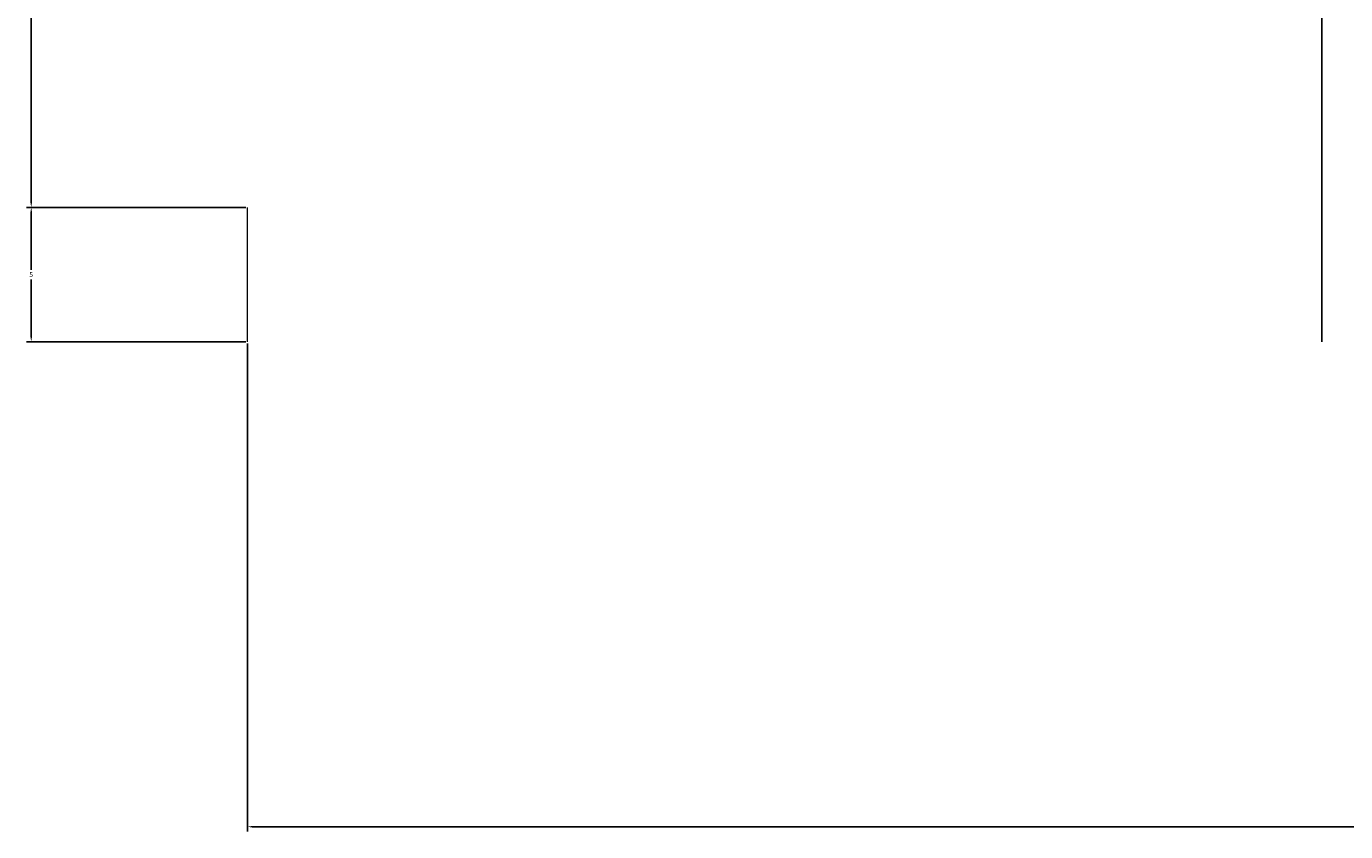
# Model space of a CAD drawing. Units: millimetres. Extents: x -48 to 129, y -118 to -41.
# Tile 1 of 6: x -48 to 1, y -118 to -88. Entities that reach past the tile are written whole.
import ezdxf

# ---------------------------------------------------------------- set-up
doc = ezdxf.new("R2010")
doc.units = ezdxf.units.MM
doc.layers.add('M-CONS', color=8, linetype='Continuous', lineweight=18)
doc.layers.add('M-DIMS', color=2, linetype='Continuous', lineweight=18)
doc.styles.get("Standard").update_dxf_attribs({"font": 'arial.ttf'})
doc.dimstyles.get("Standard").update_dxf_attribs({"dimtxt": 0.18, "dimasz": 0.18, "dimexe": 0.18, "dimexo": 0.0625, "dimgap": 0.09, "dimtad": 0, "dimtih": 1, "dimtoh": 1, "dimdec": 4, "dimzin": 0, "dimdsep": 46, "dimtxsty": 'Standard', "dimcen": 0.09, "dimadec": 0, "dimazin": 0, "dimtfac": 1, "dimtdec": 4, "dimtofl": 0, "dimtmove": 0, "dimatfit": 3, "dimfxl": 1, "dimtolj": 1, "dimtzin": 0, "dimarcsym": 0})

# ---------------------------------------------------------------- blocks, each defined once
blk = doc.blocks.new('*D1')
at = {"layer": 'Defpoints', "color": 0, "transparency": 16777216}
for p in [(120, -79.442), (-40, -99.442), (120, -117.492)]:
    blk.add_point(p, dxfattribs=at)
at = {"layer": 'M-DIMS', "color": 0, "lineweight": -2, "transparency": 16777216}
for p, q in [((120, -79.505), (120, -117.672)), ((-40, -99.505), (-40, -117.672)), ((-39.82, -117.492), (39.72, -117.492)), ((119.82, -117.492), (40.28, -117.492))]:
    blk.add_line(p, q, dxfattribs=at)
at = {"layer": 'M-DIMS', "color": 0, "transparency": 16777216}
for points in [[(-39.82, -117.462), (-39.82, -117.522), (-40, -117.492)], [(119.82, -117.462), (119.82, -117.522), (120, -117.492)]]:
    blk.add_solid(points, dxfattribs=at)
at = {"layer": 'M-DIMS', "color": 0, "transparency": 16777216, "insert": (40, -117.492), "char_height": 0.18, "attachment_point": 5}
blk.add_mtext('\\A1;160', dxfattribs=at)
blk = doc.blocks.new('*D4')
at = {"layer": 'Defpoints', "color": 0, "transparency": 16777216}
for p in [(-48.05, -94.442), (-40, -94.442), (-40, -99.442)]:
    blk.add_point(p, dxfattribs=at)
at = {"layer": 'M-DIMS', "color": 0, "lineweight": -2, "transparency": 16777216}
for p, q in [((-40.063, -94.442), (-48.23, -94.442)), ((-48.05, -94.622), (-48.05, -96.761)), ((-48.05, -99.262), (-48.05, -97.124)), ((-40.063, -99.442), (-48.23, -99.442))]:
    blk.add_line(p, q, dxfattribs=at)
at = {"layer": 'M-DIMS', "color": 0, "transparency": 16777216}
for points in [[(-48.08, -94.622), (-48.02, -94.622), (-48.05, -94.442)], [(-48.08, -99.262), (-48.02, -99.262), (-48.05, -99.442)]]:
    blk.add_solid(points, dxfattribs=at)
at = {"layer": 'M-DIMS', "color": 0, "transparency": 16777216, "insert": (-48.05, -96.942), "char_height": 0.18, "attachment_point": 5}
blk.add_mtext('\\A1;5', dxfattribs=at)
blk = doc.blocks.new('*D5')
at = {"layer": 'Defpoints', "color": 0, "transparency": 16777216}
for p in [(-48.05, -79.442), (-20, -79.442), (-40, -94.442)]:
    blk.add_point(p, dxfattribs=at)
at = {"layer": 'M-DIMS', "color": 0, "lineweight": -2, "transparency": 16777216}
for p, q in [((-20.063, -79.442), (-48.23, -79.442)), ((-48.05, -79.622), (-48.05, -86.76)), ((-48.05, -94.262), (-48.05, -87.124)), ((-40.063, -94.442), (-48.23, -94.442))]:
    blk.add_line(p, q, dxfattribs=at)
at = {"layer": 'M-DIMS', "color": 0, "transparency": 16777216}
for points in [[(-48.08, -79.622), (-48.02, -79.622), (-48.05, -79.442)], [(-48.08, -94.262), (-48.02, -94.262), (-48.05, -94.442)]]:
    blk.add_solid(points, dxfattribs=at)
at = {"layer": 'M-DIMS', "color": 0, "transparency": 16777216, "insert": (-48.05, -86.942), "char_height": 0.18, "attachment_point": 5}
blk.add_mtext('\\A1;15', dxfattribs=at)

msp = doc.modelspace()

# ---------------------------------------------------------------- linework, layer by layer
at = {"layer": 'M-CONS', "extrusion": (-1, 0, 0)}
for p, q in [((0, -59.442, 46.324), (0, -99.442, 46.324)), ((0, -79.442, 86.324), (0, -94.442, 86.324)), ((-40, -99.442, 46.324), (-40, -94.442, 46.324)), ((0, -94.442, 86.324), (0, -99.442, 46.324)), ((0, -99.442, 46.324), (0, -94.442, 46.324))]:
    msp.add_line(p, q, dxfattribs=at)
at = {"layer": 'M-CONS', "extrusion": (1, 0, 0)}
msp.add_circle((-79.442, 66.324), 15, dxfattribs=at)

# ---------------------------------------------------------------- dimensions: what is measured, and where the dimension line sits
at = {"layer": 'M-DIMS'}
for base, p1, p2, picture, middle in [((-48.05, -79.442), (-40, -94.442), (-20, -79.442), '*D5', (-48.05, -86.942)), ((-48.05, -94.442), (-40, -99.442), (-40, -94.442), '*D4', (-48.05, -96.942))]:
    dim = msp.add_linear_dim(base=base, p1=p1, p2=p2, angle=90, dimstyle='Standard', override={"dimdec": 0, "dimlfac": 1, "dimrnd": 0, "dimzin": 0, "dimdsep": 46, "dimlunit": 2}, dxfattribs=at)
    dim.commit()
    dim.dimension.update_dxf_attribs({"geometry": picture, "text_midpoint": middle})
dim = msp.add_linear_dim(base=(120, -117.492), p1=(-40, -99.442), p2=(120, -79.442), dimstyle='Standard', override={"dimdec": 0, "dimlfac": 1, "dimrnd": 0, "dimzin": 0, "dimdsep": 46, "dimlunit": 2}, dxfattribs=at)
dim.commit()
dim.dimension.update_dxf_attribs({"geometry": '*D1', "text_midpoint": (40, -117.492)})

doc.saveas('drawing.dxf')
